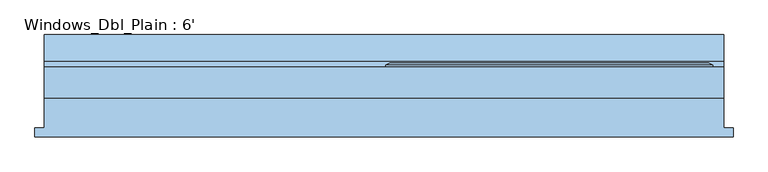
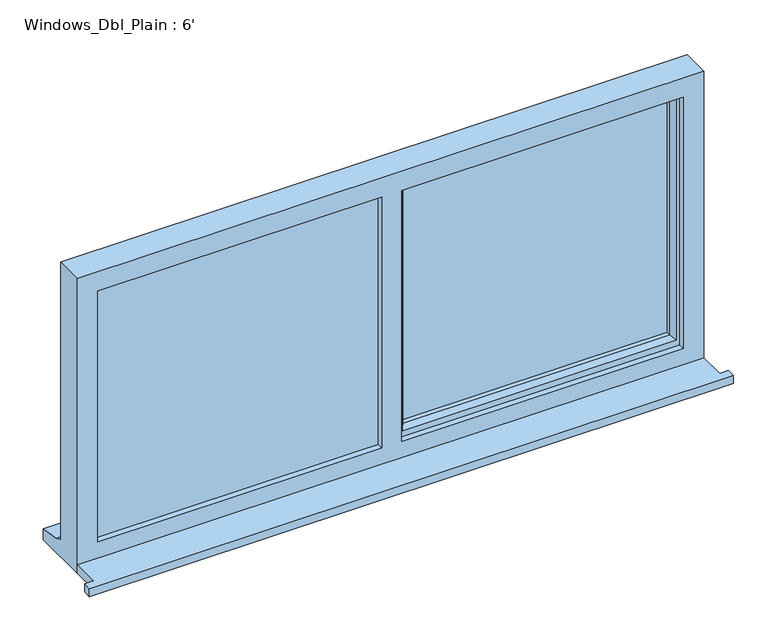
"""IFC4 building model written with IfcOpenShell, lengths in millimetres: window geometry, Windows_Dbl_Plain : 6'."""

from ifc_helpers import new_model, si_unit, frame, origin, place, context, project, spatial, polyline, outline, extrude, faceted_brep, source, transform, mapped, element, save


def windows_dbl_plain_6_3da2432f(model_context):
    return source(origin(), model_context, "Body", "SolidModel", [
        extrude(outline(polyline([(-1224.4, -123.2234322), (-1224.4, -98.2234322), (-1199.4, -98.2234322), (-1199.4, -17.8634322), (629.4, -17.8634322), (629.4, -98.2234322), (654.4, -98.2234322), (654.4, -123.2234322), (-1224.4, -123.2234322)])), frame((0.0, 0.0, 1200.0), z_axis=(0.0, 0.0, 1.0), x_axis=(1.0, 0.0, 0.0)), (0.0, 0.0, 1.0), 25.0),
        faceted_brep([(-280.0, 65.1365678, 2080.0), (-280.0, 70.9100705, 2080.0), (-280.0, 70.9100705, 1253.0), (-280.0, 65.1365678, 1253.0), (-270.0, 0.1365678, 2070.0), (-270.0, 65.1365678, 2070.0), (-270.0, 65.1365678, 1263.0), (-270.0, 0.1365678, 1263.0), (-230.0, 14.6294677, 2030.0), (-240.1480377, 0.1365678, 2040.1480377), (-240.1480377, 0.1365678, 1292.8519623), (-230.0, 14.6294677, 1303.0), (-230.0, 29.1365678, 2030.0), (-230.0, 29.1365678, 1303.0), (-240.0, 53.1365678, 2040.0), (-240.0, 29.1365678, 2040.0), (-240.0, 29.1365678, 1293.0), (-240.0, 53.1365678, 1293.0), (-230.0, 70.9100705, 2030.0), (-230.0, 53.1365678, 2030.0), (-230.0, 53.1365678, 1303.0), (-230.0, 70.9100705, 1303.0), (-247.4457548, 76.6835732, 2047.4457548), (-247.4457548, 76.6835732, 1285.5542452), (-269.2153903, 76.6835732, 2069.2153903), (-269.2153903, 76.6835732, 1263.7846097), (599.4, 70.9100705, 1253.0), (599.4, 65.1365678, 1253.0), (589.4, 65.1365678, 1263.0), (589.4, 0.1365678, 1263.0), (559.5480377, 0.1365678, 1292.8519623), (549.4, 14.6294677, 1303.0), (549.4, 29.1365678, 1303.0), (559.4, 29.1365678, 1293.0), (559.4, 53.1365678, 1293.0), (549.4, 53.1365678, 1303.0), (549.4, 70.9100705, 1303.0), (566.8457548, 76.6835732, 1285.5542452), (588.6153903, 76.6835732, 1263.7846097), (599.4, 70.9100705, 2080.0), (599.4, 65.1365678, 2080.0), (589.4, 65.1365678, 2070.0), (589.4, 0.1365678, 2070.0), (559.5480377, 0.1365678, 2040.1480377), (549.4, 14.6294677, 2030.0), (549.4, 29.1365678, 2030.0), (559.4, 29.1365678, 2040.0), (559.4, 53.1365678, 2040.0), (549.4, 53.1365678, 2030.0), (549.4, 70.9100705, 2030.0), (566.8457548, 76.6835732, 2047.4457548), (588.6153903, 76.6835732, 2069.2153903)], [[[0, 1, 2, 3]], [[4, 5, 6, 7]], [[8, 9, 10, 11]], [[12, 8, 11, 13]], [[14, 15, 16, 17]], [[18, 19, 20, 21]], [[22, 18, 21, 23]], [[1, 24, 25, 2]], [[3, 2, 26, 27]], [[7, 6, 28, 29]], [[11, 10, 30, 31]], [[13, 11, 31, 32]], [[17, 16, 33, 34]], [[21, 20, 35, 36]], [[23, 21, 36, 37]], [[2, 25, 38, 26]], [[27, 26, 39, 40]], [[29, 28, 41, 42]], [[31, 30, 43, 44]], [[32, 31, 44, 45]], [[34, 33, 46, 47]], [[36, 35, 48, 49]], [[37, 36, 49, 50]], [[26, 38, 51, 39]], [[40, 39, 1, 0]], [[3, 27, 40, 0], [5, 41, 28, 6]], [[42, 41, 5, 4]], [[7, 29, 42, 4], [9, 43, 30, 10]], [[44, 43, 9, 8]], [[45, 44, 8, 12]], [[15, 46, 33, 16], [13, 32, 45, 12]], [[47, 46, 15, 14]], [[17, 34, 47, 14], [19, 48, 35, 20]], [[49, 48, 19, 18]], [[50, 49, 18, 22]], [[24, 51, 38, 25], [23, 37, 50, 22]], [[39, 51, 24, 1]]]),
        extrude(outline(polyline([(2050.0, -310.0), (2070.0, -310.0), (2070.0, -1159.4), (1263.0, -1159.4), (1263.0, -310.0), (1283.0, -310.0), (1283.0, -1139.4), (2050.0, -1139.4), (2050.0, -310.0)])), frame((0.0, 24.1365678, 0.0), z_axis=(0.0, 1.0, 0.0), x_axis=(0.0, 0.0, 1.0)), (0.0, 0.0, 1.0), 41.0),
        faceted_brep([(629.4, -17.8634322, 2110.0), (-1199.4, -17.8634322, 2110.0), (-1199.4, -17.8634322, 1200.0), (629.4, -17.8634322, 1200.0), (569.4, -17.8634322, 2050.0), (569.4, -17.8634322, 1275.0), (-252.0, -17.8634322, 1275.0), (-252.0, -17.8634322, 2050.0), (-310.0, -17.8634322, 2050.0), (-310.0, -17.8634322, 1275.0), (-1139.4, -17.8634322, 1275.0), (-1139.4, -17.8634322, 2050.0), (-1199.4, 65.1365678, 2110.0), (-1199.4, 65.1365678, 1251.0), (-1199.4, 80.1365678, 1249.68767), (-1199.4, 80.1365678, 1244.7449676), (-1199.4, 152.6365678, 1233.8088847), (-1199.4, 152.6365678, 1200.0), (629.4, 65.1365678, 2110.0), (629.4, 65.1365678, 1251.0), (-1159.4, 65.1365678, 2070.0), (-1159.4, 65.1365678, 1263.0), (-310.0, 65.1365678, 1263.0), (-310.0, 65.1365678, 2070.0), (-270.0, 65.1365678, 2070.0), (-270.0, 65.1365678, 1263.0), (589.4, 65.1365678, 1263.0), (589.4, 65.1365678, 2070.0), (-1159.4, 0.1365678, 2070.0), (-1159.4, 0.1365678, 1263.0), (-300.0, 0.1365678, 2070.0), (-300.0, 0.1365678, 1263.0), (-310.0, 0.1365678, 2050.0), (-1139.4, 0.1365678, 2050.0), (-1139.4, 0.1365678, 1275.0), (-310.0, 0.1365678, 1275.0), (-270.0, 0.1365678, 2070.0), (589.4, 0.1365678, 2070.0), (589.4, 0.1365678, 1263.0), (-270.0, 0.1365678, 1263.0), (569.4, 0.1365678, 2050.0), (-252.0, 0.1365678, 2050.0), (-252.0, 0.1365678, 1275.0), (569.4, 0.1365678, 1275.0), (-310.0, 24.1365678, 2070.0), (-300.0, 24.1365678, 2070.0), (629.4, 152.6365678, 1200.0), (629.4, 152.6365678, 1233.8088847), (629.4, 80.1365678, 1244.7449676), (629.4, 80.1365678, 1249.68767), (-300.0, 24.1365678, 1263.0), (-310.0, 24.1365678, 1263.0)], [[[0, 1, 2, 3], [4, 5, 6, 7], [8, 9, 10, 11]], [[2, 1, 12, 13, 14, 15, 16, 17]], [[13, 12, 18, 19], [20, 21, 22, 23], [24, 25, 26, 27]], [[21, 20, 28, 29]], [[28, 30, 31, 29], [32, 33, 34, 35]], [[36, 37, 38, 39], [40, 41, 42, 43]], [[33, 11, 10, 34]], [[1, 0, 18, 12]], [[28, 20, 23, 44, 45, 30]], [[27, 37, 36, 24]], [[11, 33, 32, 8]], [[40, 4, 7, 41]], [[19, 18, 0, 3, 46, 47, 48, 49]], [[27, 26, 38, 37]], [[4, 40, 43, 5]], [[45, 50, 31, 30]], [[50, 45, 44, 51]], [[51, 44, 23, 22]], [[25, 24, 36, 39]], [[41, 7, 6, 42]], [[8, 32, 35, 9]], [[46, 3, 2, 17]], [[47, 46, 17, 16]], [[48, 47, 16, 15]], [[49, 48, 15, 14]], [[19, 49, 14, 13]], [[22, 21, 29, 31, 50, 51]], [[26, 25, 39, 38]], [[6, 5, 43, 42]], [[35, 34, 10, 9]]]),
        extrude(outline(polyline([(-1159.4, 24.1365678), (-300.0, 24.1365678), (-300.0, 0.1365678), (-1159.4, 0.1365678), (-1159.4, 24.1365678)])), frame((0.0, 0.0, 1263.0), z_axis=(0.0, 0.0, 1.0), x_axis=(1.0, 0.0, 0.0)), (0.0, 0.0, 1.0), 807.0),
        extrude(outline(polyline([(559.4, 29.1365678), (-240.0, 29.1365678), (-240.0, 53.1365678), (559.4, 53.1365678), (559.4, 29.1365678)])), frame((0.0, 0.0, 1293.0), z_axis=(0.0, 0.0, 1.0), x_axis=(1.0, 0.0, 0.0)), (0.0, 0.0, 1.0), 747.0),
    ])


if __name__ == "__main__":
    model = new_model("IFC4")
    model_context = context("Model", 3, world=origin())
    ifc_project = project(units=[si_unit("LENGTHUNIT", "METRE", prefix="MILLI")], contexts=[model_context])
    site = spatial("IfcSite", under=ifc_project)
    building = spatial("IfcBuilding", under=site)
    placement = place(None, origin())
    windows_dbl_plain_6_shape = windows_dbl_plain_6_3da2432f(model_context)
    element("IfcWindow", 1, ObjectType="Windows_Dbl_Plain : 6'", at=placement, inside=building, context=model_context, shape_type="MappedRepresentation", body=[
        mapped(windows_dbl_plain_6_shape, transform((0.0, 0.0, 0.0), x_axis=(1.0, 0.0, 0.0), y_axis=(0.0, 1.0, 0.0), z_axis=(0.0, 0.0, 1.0))),
    ])
    save(model, "model.ifc")

# Revit data of these elements
# Type "Windows_Dbl_Plain : 6'"
#   Type Mark = "62"
#   Operation = "DoublePanelVertical"
#   Construction Type Id = "GSP4R"
#   Manufacturer = "Revit"
#   Keynote = "L10"
#   Analytic Construction = "1/8 in Pilkington single glazing"
#   Wrap Layers (Ext) from Ext = 0.336286 ft
#   Wrap Layers (Int) from Ext = 0.582349 ft
#   Window Board Projection = 0.082021 ft
#   Window Board Extension = 0.082021 ft
#   Visual Light Transmittance = 0.9
#   Solar Heat Gain Coefficient = 0.78
#   Rough Width = 6.0 ft
#   Rough Height = 2.985564 ft
#   Height = 2.985564 ft
#   Width = 6.0 ft
#   Heat Transfer Coefficient (U) = 3.6886 W/(m²·K)
#   Glazing Thickness = 0.07874 ft
#   FrameOffset - External = 0.164042 ft
#   Frame Depth = 0.213255 ft
#   Default Head Height = 6.922572 ft
#   Cill Depth = 0.287073 ft
#   Cavity Closer Width = 0.164042 ft
#   Cavity Closer Offset from Ext = 0.336286 ft
#   Cavity Closer Depth = 0.278871 ft
#   Vis - Cavity Closers = yes
#   Define Thermal Properties by = 1
#   Material Trim = Window Frame
#   Material Glass = Glass
#   Material Frame = Window Frame
#   Wall Closure = (empty or 0)
# Element 1 (IfcWindow, "Windows_Dbl_Plain : 6'")
#   Materials on its faces: "Window Frame", "Glass"
# Materials
#   "Window Frame": colour RGB 249 249 249, transparency 0, Keynote = "L10", Cost = 0
#   "Glass": class "Glass", colour RGB 0 128 192, transparency 0.9, Description = "Soda Lime Glass", Cost = 0
